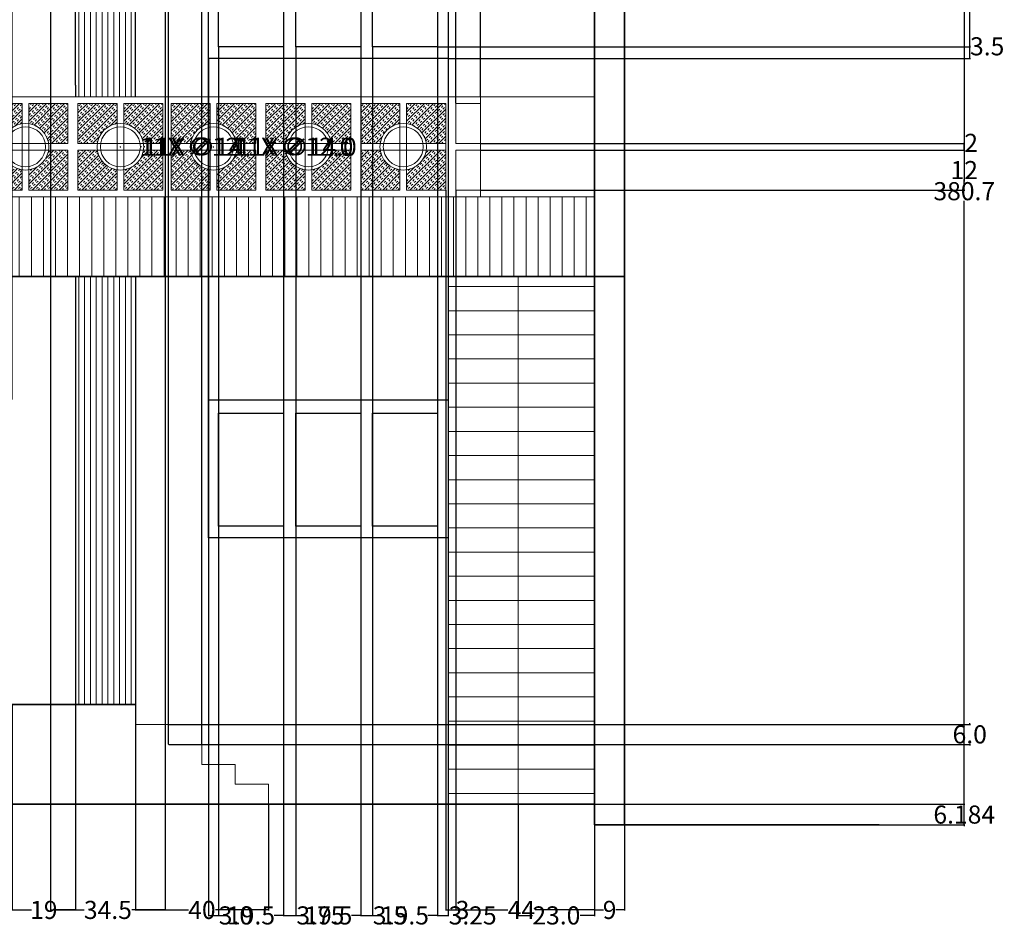
# Model space of a CAD drawing. Units: inches. Extents: x 12 to 590, y 127 to 569.
# Tile 3 of 4: x 294 to 590, y 127 to 399. Entities that reach past the tile are written whole.
import ezdxf

# ---------------------------------------------------------------- set-up
doc = ezdxf.new("R2010")
doc.units = ezdxf.units.IN
doc.header["$MEASUREMENT"] = 0
for name, color, linetype, lineweight in [('A-ANNO-DIMS', 2, 'Continuous', 18), ('A-COLS', 1, 'Continuous', 25), ('A-DETL-RAIL', 6, 'Continuous', 18), ('A-ELEV', 7, 'Continuous', 35), ('A-FLOR-STRS', 2, 'Continuous', 18), ('A-GLAZ', 4, 'Continuous', 25), ('A-WALL-PATT', 8, 'Continuous', 13)]:
    doc.layers.add(name, color=color, linetype=linetype, lineweight=lineweight)
doc.styles.get("Standard").update_dxf_attribs({"font": 'arial.ttf'})
doc.dimstyles.get("Standard").update_dxf_attribs({"dimtxt": 5.4375, "dimasz": 0.18, "dimexe": 0.18, "dimexo": 0.0625, "dimgap": 0.09, "dimtad": 0, "dimtih": 1, "dimtoh": 1, "dimdec": 4, "dimzin": 0, "dimdsep": 46, "dimlunit": 4, "dimtxsty": 'Standard', "dimcen": 0.09, "dimadec": 0, "dimazin": 0, "dimtfac": 1, "dimtdec": 4, "dimtofl": 0, "dimtmove": 0, "dimatfit": 3, "dimfxl": 1, "dimtolj": 1, "dimtzin": 0, "dimarcsym": 0})

# ---------------------------------------------------------------- blocks, each defined once
blk = doc.blocks.new('BALUSTRADE-PANEL')
for p, q in [((11.75, 13), (11.75, 26)), ((13.75, 13), (13.75, 26)), ((12.75, 14), (0, 14)), ((12.75, 12), (0, 12)), ((11.75, 13), (11.75, 0)), ((12.75, 14), (25.5, 14)), ((12.75, 12), (25.5, 12)), ((13.75, 13), (13.75, 0))]:
    blk.add_line(p, q)
for points in [[(0, 14), (0, 26), (11.75, 26)], [(13.75, 26), (25.5, 26), (25.5, 14)], [(11.75, 0), (0, 0), (0, 12)], [(25.5, 12), (25.5, 0), (13.75, 0)]]:
    blk.add_lwpolyline(points)
for radius in [7, 6]:
    blk.add_circle((12.75, 13), radius)
blk = doc.blocks.new('WIN-3PANE')
for points in [[(0, 41.5), (72, 41.5), (72, 0), (0, 0)], [(3, 37.5), (22.5, 37.5), (22.5, 3.5), (3, 3.5)], [(26.25, 37.5), (45.75, 37.5), (45.75, 3.5), (26.25, 3.5)], [(49.25, 37.5), (68.75, 37.5), (68.75, 3.5), (49.25, 3.5)]]:
    blk.add_lwpolyline(points, close=True)
blk = doc.blocks.new('*D8')
at = {"layer": 'A-ANNO-DIMS', "color": 0, "lineweight": -2, "transparency": 16777216}
for p, q in [((475.56, 538), (577.73, 538)), ((577.55, 537.82), (577.55, 350.53)), ((577.55, 157.5), (577.55, 344.79)), ((475.56, 157.32), (577.73, 157.32))]:
    blk.add_line(p, q, dxfattribs=at)
at = {"layer": 'A-ANNO-DIMS', "color": 0, "transparency": 16777216}
for points in [[(577.52, 537.82), (577.58, 537.82), (577.55, 538)], [(577.52, 157.5), (577.58, 157.5), (577.55, 157.32)]]:
    blk.add_solid(points, dxfattribs=at)
at = {"layer": 'Defpoints', "color": 0, "transparency": 16777216}
for p in [(475.5, 538), (475.5, 157.32), (577.55, 157.32)]:
    blk.add_point(p, dxfattribs=at)
at = {"layer": 'A-ANNO-DIMS', "color": 0, "transparency": 16777216, "insert": (577.55, 347.66), "char_height": 5.438, "attachment_point": 5}
blk.add_mtext('\\A1;380.7', dxfattribs=at)
blk = doc.blocks.new('*D15')
at = {"layer": 'A-ANNO-DIMS', "color": 0, "lineweight": -2, "transparency": 16777216}
for p, q in [((466.56, 163.5), (577.73, 163.5)), ((577.55, 163.68), (577.55, 163.86)), ((475.56, 157.32), (577.73, 157.32)), ((577.55, 157.14), (577.55, 156.96))]:
    blk.add_line(p, q, dxfattribs=at)
at = {"layer": 'A-ANNO-DIMS', "color": 0, "transparency": 16777216}
for points in [[(577.52, 163.68), (577.58, 163.68), (577.55, 163.5)], [(577.52, 157.14), (577.58, 157.14), (577.55, 157.32)]]:
    blk.add_solid(points, dxfattribs=at)
at = {"layer": 'Defpoints', "color": 0, "transparency": 16777216}
for p in [(466.5, 163.5), (577.55, 163.5), (475.5, 157.32)]:
    blk.add_point(p, dxfattribs=at)
at = {"layer": 'A-ANNO-DIMS', "color": 0, "transparency": 16777216, "insert": (577.55, 160.41), "char_height": 5.438, "attachment_point": 5}
blk.add_mtext('\\A1;6.184', dxfattribs=at)
blk = doc.blocks.new('*D24')
at = {"layer": 'A-ANNO-DIMS', "color": 0, "lineweight": -2, "transparency": 16777216}
for p, q in [((291.5, 193.44), (291.5, 131.59)), ((310.5, 193.44), (310.5, 131.59)), ((291.68, 131.77), (297.27, 131.77)), ((310.32, 131.77), (304.73, 131.77))]:
    blk.add_line(p, q, dxfattribs=at)
at = {"layer": 'A-ANNO-DIMS', "color": 0, "transparency": 16777216}
for points in [[(291.68, 131.8), (291.68, 131.74), (291.5, 131.77)], [(310.32, 131.8), (310.32, 131.74), (310.5, 131.77)]]:
    blk.add_solid(points, dxfattribs=at)
at = {"layer": 'Defpoints', "color": 0, "transparency": 16777216}
for p in [(291.5, 193.5), (310.5, 193.5), (310.5, 131.77)]:
    blk.add_point(p, dxfattribs=at)
at = {"layer": 'A-ANNO-DIMS', "color": 0, "transparency": 16777216, "insert": (301, 131.77), "char_height": 5.438, "attachment_point": 5}
blk.add_mtext('\\A1;19', dxfattribs=at)
blk = doc.blocks.new('*D25')
at = {"layer": 'A-ANNO-DIMS', "color": 0, "lineweight": -2, "transparency": 16777216}
for p, q in [((328.5, 193.44), (328.5, 131.59)), ((368.5, 163.44), (368.5, 131.59)), ((328.68, 131.77), (344.42, 131.77)), ((368.32, 131.77), (352.58, 131.77))]:
    blk.add_line(p, q, dxfattribs=at)
at = {"layer": 'A-ANNO-DIMS', "color": 0, "transparency": 16777216}
for points in [[(328.68, 131.8), (328.68, 131.74), (328.5, 131.77)], [(368.32, 131.8), (368.32, 131.74), (368.5, 131.77)]]:
    blk.add_solid(points, dxfattribs=at)
at = {"layer": 'Defpoints', "color": 0, "transparency": 16777216}
for p in [(328.5, 193.5), (368.5, 163.5), (368.5, 131.77)]:
    blk.add_point(p, dxfattribs=at)
at = {"layer": 'A-ANNO-DIMS', "color": 0, "transparency": 16777216, "insert": (348.5, 131.77), "char_height": 5.438, "attachment_point": 5}
blk.add_mtext('\\A1;40', dxfattribs=at)
blk = doc.blocks.new('*D26')
at = {"layer": 'A-ANNO-DIMS', "color": 0, "lineweight": -2, "transparency": 16777216}
for p, q in [((422.5, 243.44), (422.5, 131.59)), ((466.5, 163.44), (466.5, 131.59)), ((422.68, 131.77), (440.42, 131.77)), ((466.32, 131.77), (448.58, 131.77))]:
    blk.add_line(p, q, dxfattribs=at)
at = {"layer": 'A-ANNO-DIMS', "color": 0, "transparency": 16777216}
for points in [[(422.68, 131.8), (422.68, 131.74), (422.5, 131.77)], [(466.32, 131.8), (466.32, 131.74), (466.5, 131.77)]]:
    blk.add_solid(points, dxfattribs=at)
at = {"layer": 'Defpoints', "color": 0, "transparency": 16777216}
for p in [(422.5, 243.5), (466.5, 163.5), (466.5, 131.77)]:
    blk.add_point(p, dxfattribs=at)
at = {"layer": 'A-ANNO-DIMS', "color": 0, "transparency": 16777216, "insert": (444.5, 131.77), "char_height": 5.438, "attachment_point": 5}
blk.add_mtext('\\A1;44', dxfattribs=at)
blk = doc.blocks.new('*D27')
at = {"layer": 'A-ANNO-DIMS', "color": 0, "lineweight": -2, "transparency": 16777216}
for p, q in [((466.5, 163.44), (466.5, 131.59)), ((475.5, 157.25), (475.5, 131.59)), ((466.68, 131.77), (469.12, 131.77)), ((475.32, 131.77), (472.88, 131.77))]:
    blk.add_line(p, q, dxfattribs=at)
at = {"layer": 'A-ANNO-DIMS', "color": 0, "transparency": 16777216}
for points in [[(466.68, 131.8), (466.68, 131.74), (466.5, 131.77)], [(475.32, 131.8), (475.32, 131.74), (475.5, 131.77)]]:
    blk.add_solid(points, dxfattribs=at)
at = {"layer": 'Defpoints', "color": 0, "transparency": 16777216}
for p in [(466.5, 163.5), (475.5, 157.32), (475.5, 131.77)]:
    blk.add_point(p, dxfattribs=at)
at = {"layer": 'A-ANNO-DIMS', "color": 0, "transparency": 16777216, "insert": (471, 131.77), "char_height": 5.438, "attachment_point": 5}
blk.add_mtext('\\A1;9', dxfattribs=at)
blk = doc.blocks.new('*D40')
at = {"layer": 'A-ANNO-DIMS', "color": 0, "lineweight": -2, "transparency": 16777216}
for p, q in [((303, 455.94), (303, 131.59)), ((337.5, 455.94), (337.5, 131.59)), ((303.18, 131.77), (313.08, 131.77)), ((337.32, 131.77), (327.42, 131.77))]:
    blk.add_line(p, q, dxfattribs=at)
at = {"layer": 'A-ANNO-DIMS', "color": 0, "transparency": 16777216}
for points in [[(303.18, 131.8), (303.18, 131.74), (303, 131.77)], [(337.32, 131.8), (337.32, 131.74), (337.5, 131.77)]]:
    blk.add_solid(points, dxfattribs=at)
at = {"layer": 'Defpoints', "color": 0, "transparency": 16777216}
for p in [(303, 456), (337.5, 456), (337.5, 131.77)]:
    blk.add_point(p, dxfattribs=at)
at = {"layer": 'A-ANNO-DIMS', "color": 0, "transparency": 16777216, "insert": (320.25, 131.77), "char_height": 5.438, "attachment_point": 5}
blk.add_mtext('\\A1;34.5', dxfattribs=at)
blk = doc.blocks.new('*D48')
at = {"layer": 'A-ANNO-DIMS', "color": 0, "lineweight": -2, "transparency": 16777216}
for p, q in [((421.75, 347.94), (421.75, 131.59)), ((424.75, 347.94), (424.75, 131.59)), ((421.93, 131.77), (424.57, 131.77)), ((424.75, 131.77), (424.93, 131.77))]:
    blk.add_line(p, q, dxfattribs=at)
at = {"layer": 'A-ANNO-DIMS', "color": 0, "transparency": 16777216}
for points in [[(421.93, 131.8), (421.93, 131.74), (421.75, 131.77)], [(424.57, 131.8), (424.57, 131.74), (424.75, 131.77)]]:
    blk.add_solid(points, dxfattribs=at)
at = {"layer": 'Defpoints', "color": 0, "transparency": 16777216}
for p in [(421.75, 348), (424.75, 348), (424.75, 131.77)]:
    blk.add_point(p, dxfattribs=at)
at = {"layer": 'A-ANNO-DIMS', "color": 0, "transparency": 16777216, "insert": (426.8, 131.77), "char_height": 5.438, "attachment_point": 5}
blk.add_mtext('\\A1;3', dxfattribs=at)
blk = doc.blocks.new('*D49')
at = {"layer": 'A-ANNO-DIMS', "color": 0, "lineweight": -2, "transparency": 16777216}
for p, q in [((424.75, 374.06), (424.75, 563.73)), ((424.93, 563.55), (432.07, 563.55)), ((432.25, 376.06), (432.25, 563.73)), ((432.25, 563.55), (432.43, 563.55))]:
    blk.add_line(p, q, dxfattribs=at)
at = {"layer": 'A-ANNO-DIMS', "color": 0, "transparency": 16777216}
for points in [[(424.93, 563.58), (424.93, 563.52), (424.75, 563.55)], [(432.07, 563.58), (432.07, 563.52), (432.25, 563.55)]]:
    blk.add_solid(points, dxfattribs=at)
at = {"layer": 'Defpoints', "color": 0, "transparency": 16777216}
for p in [(432.25, 563.55), (432.25, 376), (424.75, 374)]:
    blk.add_point(p, dxfattribs=at)
at = {"layer": 'A-ANNO-DIMS', "color": 0, "transparency": 16777216, "insert": (437.47, 563.55), "char_height": 5.438, "attachment_point": 5}
blk.add_mtext('\\A1;7.5', dxfattribs=at)
blk = doc.blocks.new('*D50')
at = {"layer": 'A-ANNO-DIMS', "color": 0, "lineweight": -2, "transparency": 16777216}
for p, q in [((432.25, 376.06), (432.25, 563.73)), ((432.43, 563.55), (440.09, 563.55)), ((466.32, 563.55), (458.66, 563.55)), ((466.5, 376.06), (466.5, 563.73))]:
    blk.add_line(p, q, dxfattribs=at)
at = {"layer": 'A-ANNO-DIMS', "color": 0, "transparency": 16777216}
for points in [[(432.43, 563.58), (432.43, 563.52), (432.25, 563.55)], [(466.32, 563.58), (466.32, 563.52), (466.5, 563.55)]]:
    blk.add_solid(points, dxfattribs=at)
at = {"layer": 'Defpoints', "color": 0, "transparency": 16777216}
for p in [(466.5, 563.55), (432.25, 376), (466.5, 376)]:
    blk.add_point(p, dxfattribs=at)
at = {"layer": 'A-ANNO-DIMS', "color": 0, "transparency": 16777216, "insert": (449.38, 563.55), "char_height": 5.438, "attachment_point": 5}
blk.add_mtext('\\A1;34.25', dxfattribs=at)
blk = doc.blocks.new('*D51')
at = {"layer": 'A-ANNO-DIMS', "color": 0, "lineweight": -2, "transparency": 16777216}
for p, q in [((432.31, 360), (577.73, 360)), ((577.55, 359.82), (577.55, 356.82)), ((577.55, 348.18), (577.55, 351.18)), ((432.31, 348), (577.73, 348))]:
    blk.add_line(p, q, dxfattribs=at)
at = {"layer": 'A-ANNO-DIMS', "color": 0, "transparency": 16777216}
for points in [[(577.52, 359.82), (577.58, 359.82), (577.55, 360)], [(577.52, 348.18), (577.58, 348.18), (577.55, 348)]]:
    blk.add_solid(points, dxfattribs=at)
at = {"layer": 'Defpoints', "color": 0, "transparency": 16777216}
for p in [(432.25, 360), (577.55, 360), (432.25, 348)]:
    blk.add_point(p, dxfattribs=at)
at = {"layer": 'A-ANNO-DIMS', "color": 0, "transparency": 16777216, "insert": (577.55, 354), "char_height": 5.438, "attachment_point": 5}
blk.add_mtext('\\A1;12', dxfattribs=at)
blk = doc.blocks.new('*D52')
at = {"layer": 'A-ANNO-DIMS', "color": 0, "lineweight": -2, "transparency": 16777216}
for p, q in [((432.31, 362), (577.73, 362)), ((577.55, 362), (577.55, 362.18)), ((577.55, 362.18), (577.73, 362.18)), ((577.55, 360.18), (577.55, 361.82)), ((432.31, 360), (577.73, 360))]:
    blk.add_line(p, q, dxfattribs=at)
at = {"layer": 'A-ANNO-DIMS', "color": 0, "transparency": 16777216}
for points in [[(577.52, 361.82), (577.58, 361.82), (577.55, 362)], [(577.52, 360.18), (577.58, 360.18), (577.55, 360)]]:
    blk.add_solid(points, dxfattribs=at)
at = {"layer": 'Defpoints', "color": 0, "transparency": 16777216}
for p in [(432.25, 362), (577.55, 362), (432.25, 360)]:
    blk.add_point(p, dxfattribs=at)
at = {"layer": 'A-ANNO-DIMS', "color": 0, "transparency": 16777216, "insert": (579.62, 362.18), "char_height": 5.438, "attachment_point": 5}
blk.add_mtext('\\A1;2', dxfattribs=at)
blk = doc.blocks.new('*D54')
at = {"layer": 'A-ANNO-DIMS', "color": 0, "lineweight": -2, "transparency": 16777216}
for p, q in [((323.91, 361), (324.09, 361)), ((324, 360.91), (324, 361.09)), ((331.36, 361), (331.18, 361))]:
    blk.add_line(p, q, dxfattribs=at)
at = {"layer": 'A-ANNO-DIMS', "color": 0, "transparency": 16777216}
blk.add_solid([(331.18, 361.03), (331.18, 360.97), (331, 361)], dxfattribs=at)
at = {"layer": 'Defpoints', "color": 0, "transparency": 16777216}
for p in [(317, 361), (331, 361)]:
    blk.add_point(p, dxfattribs=at)
at = {"layer": 'A-ANNO-DIMS', "color": 0, "transparency": 16777216, "insert": (345.84, 361), "char_height": 5.4375, "attachment_point": 5}
blk.add_mtext('\\A1;11X ∅14', dxfattribs=at)
blk = doc.blocks.new('*D55')
at = {"layer": 'A-ANNO-DIMS', "color": 0, "lineweight": -2, "transparency": 16777216}
for p, q in [((323.91, 361), (324.09, 361)), ((324, 360.91), (324, 361.09)), ((330.36, 361), (330.18, 361))]:
    blk.add_line(p, q, dxfattribs=at)
at = {"layer": 'A-ANNO-DIMS', "color": 0, "transparency": 16777216}
blk.add_solid([(330.18, 361.03), (330.18, 360.97), (330, 361)], dxfattribs=at)
at = {"layer": 'Defpoints', "color": 0, "transparency": 16777216}
for p in [(318, 361), (330, 361)]:
    blk.add_point(p, dxfattribs=at)
at = {"layer": 'A-ANNO-DIMS', "color": 0, "transparency": 16777216, "insert": (344.83, 361), "char_height": 5.4375, "attachment_point": 5}
blk.add_mtext('\\A1;11X ∅12', dxfattribs=at)
blk = doc.blocks.new('*D60')
at = {"layer": 'A-ANNO-DIMS', "color": 0, "lineweight": -2, "transparency": 16777216}
for p, q in [((291.5, 285.06), (291.5, 565.38)), ((291.68, 565.2), (313.86, 565.2)), ((350.32, 565.2), (328.14, 565.2)), ((350.5, 285.06), (350.5, 565.38))]:
    blk.add_line(p, q, dxfattribs=at)
at = {"layer": 'A-ANNO-DIMS', "color": 0, "transparency": 16777216}
for points in [[(291.68, 565.23), (291.68, 565.17), (291.5, 565.2)], [(350.32, 565.23), (350.32, 565.17), (350.5, 565.2)]]:
    blk.add_solid(points, dxfattribs=at)
at = {"layer": 'Defpoints', "color": 0, "transparency": 16777216}
for p in [(350.5, 565.2), (291.5, 285), (350.5, 285)]:
    blk.add_point(p, dxfattribs=at)
at = {"layer": 'A-ANNO-DIMS', "color": 0, "transparency": 16777216, "insert": (321, 565.2), "char_height": 5.438, "attachment_point": 5}
blk.add_mtext('\\A1;59.0', dxfattribs=at)
blk = doc.blocks.new('*D61')
at = {"layer": 'A-ANNO-DIMS', "color": 0, "lineweight": -2, "transparency": 16777216}
for p, q in [((338.5625, 187.5), (579.38, 187.5)), ((579.2, 187.68), (579.2, 187.86)), ((338.5625, 181.5), (579.38, 181.5)), ((579.2, 181.32), (579.2, 181.14))]:
    blk.add_line(p, q, dxfattribs=at)
at = {"layer": 'A-ANNO-DIMS', "color": 0, "transparency": 16777216}
for points in [[(579.17, 187.68), (579.23, 187.68), (579.2, 187.5)], [(579.17, 181.32), (579.23, 181.32), (579.2, 181.5)]]:
    blk.add_solid(points, dxfattribs=at)
at = {"layer": 'Defpoints', "color": 0, "transparency": 16777216}
for p in [(338.5, 187.5), (338.5, 181.5), (579.2, 181.5)]:
    blk.add_point(p, dxfattribs=at)
at = {"layer": 'A-ANNO-DIMS', "color": 0, "transparency": 16777216, "insert": (579.2, 184.5), "char_height": 5.4375, "attachment_point": 5}
blk.add_mtext('\\A1;6.0', dxfattribs=at)
blk = doc.blocks.new('*D62')
at = {"layer": 'A-ANNO-DIMS', "color": 0, "lineweight": -2, "transparency": 16777216}
for p, q in [((338.5, 181.5625), (338.5, 565.38)), ((338.68, 565.2), (348.32, 565.2)), ((348.5, 181.5625), (348.5, 565.38)), ((348.5, 565.2), (348.68, 565.2))]:
    blk.add_line(p, q, dxfattribs=at)
at = {"layer": 'A-ANNO-DIMS', "color": 0, "transparency": 16777216}
for points in [[(338.68, 565.23), (338.68, 565.17), (338.5, 565.2)], [(348.32, 565.23), (348.32, 565.17), (348.5, 565.2)]]:
    blk.add_solid(points, dxfattribs=at)
at = {"layer": 'Defpoints', "color": 0, "transparency": 16777216}
for p in [(348.5, 565.2), (338.5, 181.5), (348.5, 181.5)]:
    blk.add_point(p, dxfattribs=at)
at = {"layer": 'A-ANNO-DIMS', "color": 0, "transparency": 16777216, "insert": (355.566875, 565.2), "char_height": 5.4375, "attachment_point": 5}
blk.add_mtext('\\A1;10.0', dxfattribs=at)
blk = doc.blocks.new('*D63')
at = {"layer": 'A-ANNO-DIMS', "color": 0, "lineweight": -2, "transparency": 16777216}
for p, q in [((443.5, 163.44), (443.5, 129.94)), ((466.5, 163.44), (466.5, 129.94)), ((443.68, 130.12), (447.81, 130.12)), ((466.32, 130.12), (462.19, 130.12))]:
    blk.add_line(p, q, dxfattribs=at)
at = {"layer": 'A-ANNO-DIMS', "color": 0, "transparency": 16777216}
for points in [[(443.68, 130.15), (443.68, 130.09), (443.5, 130.12)], [(466.32, 130.15), (466.32, 130.09), (466.5, 130.12)]]:
    blk.add_solid(points, dxfattribs=at)
at = {"layer": 'Defpoints', "color": 0, "transparency": 16777216}
for p in [(443.5, 163.5), (466.5, 163.5), (466.5, 130.12)]:
    blk.add_point(p, dxfattribs=at)
at = {"layer": 'A-ANNO-DIMS', "color": 0, "transparency": 16777216, "insert": (455, 130.12), "char_height": 5.438, "attachment_point": 5}
blk.add_mtext('\\A1;23.0', dxfattribs=at)
blk = doc.blocks.new('*D64')
at = {"layer": 'A-ANNO-DIMS', "color": 0, "lineweight": -2, "transparency": 16777216}
for p, q in [((353.5, 390.94), (353.5, 129.94)), ((350.5, 387.44), (350.5, 129.94)), ((350.68, 130.12), (353.32, 130.12)), ((353.5, 130.12), (353.68, 130.12))]:
    blk.add_line(p, q, dxfattribs=at)
at = {"layer": 'A-ANNO-DIMS', "color": 0, "transparency": 16777216}
for points in [[(350.68, 130.15), (350.68, 130.09), (350.5, 130.12)], [(353.32, 130.15), (353.32, 130.09), (353.5, 130.12)]]:
    blk.add_solid(points, dxfattribs=at)
at = {"layer": 'Defpoints', "color": 0, "transparency": 16777216}
for p in [(353.5, 391), (350.5, 387.5), (353.5, 130.12)]:
    blk.add_point(p, dxfattribs=at)
at = {"layer": 'A-ANNO-DIMS', "color": 0, "transparency": 16777216, "insert": (358.71, 130.12), "char_height": 5.438, "attachment_point": 5}
blk.add_mtext('\\A1;3.0', dxfattribs=at)
blk = doc.blocks.new('*D65')
at = {"layer": 'A-ANNO-DIMS', "color": 0, "lineweight": -2, "transparency": 16777216}
for p, q in [((353.5, 390.94), (353.5, 129.94)), ((373, 390.94), (373, 129.94)), ((353.68, 130.12), (356.33, 130.12)), ((372.82, 130.12), (370.17, 130.12))]:
    blk.add_line(p, q, dxfattribs=at)
at = {"layer": 'A-ANNO-DIMS', "color": 0, "transparency": 16777216}
for points in [[(353.68, 130.15), (353.68, 130.09), (353.5, 130.12)], [(372.82, 130.15), (372.82, 130.09), (373, 130.12)]]:
    blk.add_solid(points, dxfattribs=at)
at = {"layer": 'Defpoints', "color": 0, "transparency": 16777216}
for p in [(353.5, 391), (373, 391), (373, 130.12)]:
    blk.add_point(p, dxfattribs=at)
at = {"layer": 'A-ANNO-DIMS', "color": 0, "transparency": 16777216, "insert": (363.25, 130.12), "char_height": 5.438, "attachment_point": 5}
blk.add_mtext('\\A1;19.5', dxfattribs=at)
blk = doc.blocks.new('*D66')
at = {"layer": 'A-ANNO-DIMS', "color": 0, "lineweight": -2, "transparency": 16777216}
for p, q in [((373, 390.94), (373, 129.94)), ((376.75, 390.94), (376.75, 129.94)), ((373.18, 130.12), (376.57, 130.12)), ((376.75, 130.12), (376.93, 130.12))]:
    blk.add_line(p, q, dxfattribs=at)
at = {"layer": 'A-ANNO-DIMS', "color": 0, "transparency": 16777216}
for points in [[(373.18, 130.15), (373.18, 130.09), (373, 130.12)], [(376.57, 130.15), (376.57, 130.09), (376.75, 130.12)]]:
    blk.add_solid(points, dxfattribs=at)
at = {"layer": 'Defpoints', "color": 0, "transparency": 16777216}
for p in [(373, 391), (376.75, 391), (376.75, 130.12)]:
    blk.add_point(p, dxfattribs=at)
at = {"layer": 'A-ANNO-DIMS', "color": 0, "transparency": 16777216, "insert": (384.1, 130.12), "char_height": 5.438, "attachment_point": 5}
blk.add_mtext('\\A1;3.75', dxfattribs=at)
blk = doc.blocks.new('*D67')
at = {"layer": 'A-ANNO-DIMS', "color": 0, "lineweight": -2, "transparency": 16777216}
for p, q in [((376.75, 390.94), (376.75, 129.94)), ((396.25, 390.94), (396.25, 129.94)), ((376.93, 130.12), (379.58, 130.12)), ((396.07, 130.12), (393.42, 130.12))]:
    blk.add_line(p, q, dxfattribs=at)
at = {"layer": 'A-ANNO-DIMS', "color": 0, "transparency": 16777216}
for points in [[(376.93, 130.15), (376.93, 130.09), (376.75, 130.12)], [(396.07, 130.15), (396.07, 130.09), (396.25, 130.12)]]:
    blk.add_solid(points, dxfattribs=at)
at = {"layer": 'Defpoints', "color": 0, "transparency": 16777216}
for p in [(376.75, 391), (396.25, 391), (396.25, 130.12)]:
    blk.add_point(p, dxfattribs=at)
at = {"layer": 'A-ANNO-DIMS', "color": 0, "transparency": 16777216, "insert": (386.5, 130.12), "char_height": 5.438, "attachment_point": 5}
blk.add_mtext('\\A1;19.5', dxfattribs=at)
blk = doc.blocks.new('*D68')
at = {"layer": 'A-ANNO-DIMS', "color": 0, "lineweight": -2, "transparency": 16777216}
for p, q in [((396.25, 390.94), (396.25, 129.94)), ((399.75, 390.94), (399.75, 129.94)), ((396.43, 130.12), (399.57, 130.12)), ((399.75, 130.12), (399.93, 130.12))]:
    blk.add_line(p, q, dxfattribs=at)
at = {"layer": 'A-ANNO-DIMS', "color": 0, "transparency": 16777216}
for points in [[(396.43, 130.15), (396.43, 130.09), (396.25, 130.12)], [(399.57, 130.15), (399.57, 130.09), (399.75, 130.12)]]:
    blk.add_solid(points, dxfattribs=at)
at = {"layer": 'Defpoints', "color": 0, "transparency": 16777216}
for p in [(396.25, 391), (399.75, 391), (399.75, 130.12)]:
    blk.add_point(p, dxfattribs=at)
at = {"layer": 'A-ANNO-DIMS', "color": 0, "transparency": 16777216, "insert": (404.99, 130.12), "char_height": 5.438, "attachment_point": 5}
blk.add_mtext('\\A1;3.5', dxfattribs=at)
blk = doc.blocks.new('*D69')
at = {"layer": 'A-ANNO-DIMS', "color": 0, "lineweight": -2, "transparency": 16777216}
for p, q in [((399.75, 390.94), (399.75, 129.94)), ((419.25, 390.94), (419.25, 129.94)), ((399.93, 130.12), (402.58, 130.12)), ((419.07, 130.12), (416.42, 130.12))]:
    blk.add_line(p, q, dxfattribs=at)
at = {"layer": 'A-ANNO-DIMS', "color": 0, "transparency": 16777216}
for points in [[(399.93, 130.15), (399.93, 130.09), (399.75, 130.12)], [(419.07, 130.15), (419.07, 130.09), (419.25, 130.12)]]:
    blk.add_solid(points, dxfattribs=at)
at = {"layer": 'Defpoints', "color": 0, "transparency": 16777216}
for p in [(399.75, 391), (419.25, 391), (419.25, 130.12)]:
    blk.add_point(p, dxfattribs=at)
at = {"layer": 'A-ANNO-DIMS', "color": 0, "transparency": 16777216, "insert": (409.5, 130.12), "char_height": 5.438, "attachment_point": 5}
blk.add_mtext('\\A1;19.5', dxfattribs=at)
blk = doc.blocks.new('*D70')
at = {"layer": 'A-ANNO-DIMS', "color": 0, "lineweight": -2, "transparency": 16777216}
for p, q in [((419.25, 390.94), (419.25, 129.94)), ((422.5, 387.44), (422.5, 129.94)), ((419.43, 130.12), (422.32, 130.12)), ((422.5, 130.12), (422.68, 130.12))]:
    blk.add_line(p, q, dxfattribs=at)
at = {"layer": 'A-ANNO-DIMS', "color": 0, "transparency": 16777216}
for points in [[(419.43, 130.15), (419.43, 130.09), (419.25, 130.12)], [(422.32, 130.15), (422.32, 130.09), (422.5, 130.12)]]:
    blk.add_solid(points, dxfattribs=at)
at = {"layer": 'Defpoints', "color": 0, "transparency": 16777216}
for p in [(419.25, 391), (422.5, 387.5), (422.5, 130.12)]:
    blk.add_point(p, dxfattribs=at)
at = {"layer": 'A-ANNO-DIMS', "color": 0, "transparency": 16777216, "insert": (429.85, 130.12), "char_height": 5.438, "attachment_point": 5}
blk.add_mtext('\\A1;3.25', dxfattribs=at)
blk = doc.blocks.new('*D71')
at = {"layer": 'A-ANNO-DIMS', "color": 0, "lineweight": -2, "transparency": 16777216}
for p, q in [((419.31, 391), (579.38, 391)), ((579.2, 391), (579.2, 391.18)), ((579.2, 391.18), (579.38, 391.18)), ((579.2, 387.68), (579.2, 390.82)), ((422.56, 387.5), (579.38, 387.5))]:
    blk.add_line(p, q, dxfattribs=at)
at = {"layer": 'A-ANNO-DIMS', "color": 0, "transparency": 16777216}
for points in [[(579.17, 390.82), (579.23, 390.82), (579.2, 391)], [(579.17, 387.68), (579.23, 387.68), (579.2, 387.5)]]:
    blk.add_solid(points, dxfattribs=at)
at = {"layer": 'Defpoints', "color": 0, "transparency": 16777216}
for p in [(419.25, 391), (579.2, 391), (422.5, 387.5)]:
    blk.add_point(p, dxfattribs=at)
at = {"layer": 'A-ANNO-DIMS', "color": 0, "transparency": 16777216, "insert": (584.44, 391.18), "char_height": 5.438, "attachment_point": 5}
blk.add_mtext('\\A1;3.5', dxfattribs=at)
blk = doc.blocks.new('*D72')
at = {"layer": 'A-ANNO-DIMS', "color": 0, "lineweight": -2, "transparency": 16777216}
for p, q in [((419.31, 425), (579.38, 425)), ((579.2, 424.82), (579.2, 410.87)), ((579.2, 391.18), (579.2, 405.13)), ((419.31, 391), (579.38, 391))]:
    blk.add_line(p, q, dxfattribs=at)
at = {"layer": 'A-ANNO-DIMS', "color": 0, "transparency": 16777216}
for points in [[(579.17, 424.82), (579.23, 424.82), (579.2, 425)], [(579.17, 391.18), (579.23, 391.18), (579.2, 391)]]:
    blk.add_solid(points, dxfattribs=at)
at = {"layer": 'Defpoints', "color": 0, "transparency": 16777216}
for p in [(419.25, 425), (579.2, 425), (419.25, 391)]:
    blk.add_point(p, dxfattribs=at)
at = {"layer": 'A-ANNO-DIMS', "color": 0, "transparency": 16777216, "insert": (579.2, 408), "char_height": 5.438, "attachment_point": 5}
blk.add_mtext('\\A1;34.0', dxfattribs=at)
blk = doc.blocks.new('*D74')
at = {"layer": 'A-ANNO-DIMS', "color": 0, "lineweight": -2, "transparency": 16777216}
for p, q in [((351.91, 361), (352.09, 361)), ((352, 360.91), (352, 361.09)), ((359.36, 361), (359.18, 361))]:
    blk.add_line(p, q, dxfattribs=at)
at = {"layer": 'A-ANNO-DIMS', "color": 0, "transparency": 16777216}
blk.add_solid([(359.18, 361.03), (359.18, 360.97), (359, 361)], dxfattribs=at)
at = {"layer": 'Defpoints', "color": 0, "transparency": 16777216}
for p in [(345, 361), (359, 361)]:
    blk.add_point(p, dxfattribs=at)
at = {"layer": 'A-ANNO-DIMS', "color": 0, "transparency": 16777216, "insert": (377.01, 361), "char_height": 5.4375, "attachment_point": 5}
blk.add_mtext('\\A1;11X ∅14.0', dxfattribs=at)
blk = doc.blocks.new('*D75')
at = {"layer": 'A-ANNO-DIMS', "color": 0, "lineweight": -2, "transparency": 16777216}
for p, q in [((351.91, 361), (352.09, 361)), ((352, 360.91), (352, 361.09)), ((358.36, 361), (358.18, 361))]:
    blk.add_line(p, q, dxfattribs=at)
at = {"layer": 'A-ANNO-DIMS', "color": 0, "transparency": 16777216}
blk.add_solid([(358.18, 361.03), (358.18, 360.97), (358, 361)], dxfattribs=at)
at = {"layer": 'Defpoints', "color": 0, "transparency": 16777216}
for p in [(346, 361), (358, 361)]:
    blk.add_point(p, dxfattribs=at)
at = {"layer": 'A-ANNO-DIMS', "color": 0, "transparency": 16777216, "insert": (376.01, 361), "char_height": 5.4375, "attachment_point": 5}
blk.add_mtext('\\A1;11X ∅12.0', dxfattribs=at)

msp = doc.modelspace()

# ---------------------------------------------------------------- hatches: boundary and pattern name
at = {"layer": 'A-WALL-PATT'}
h = msp.add_hatch(dxfattribs=at)
h.set_pattern_fill('ANSI31', color=256, scale=14, angle=45)
h.paths.add_polyline_path([(328.5, 456), (310.5, 456), (310.5, 379.5), (310.5, 376), (328.5, 376)])
h.paths.add_polyline_path([(328.5, 322), (310.5, 322), (310.5, 193.5), (328.5, 193.5)])
h = msp.add_hatch(dxfattribs=at)
h.set_pattern_fill('INSUL', color=256, scale=5.1, angle=45)
h.set_pattern_definition([(45, (171.25, 0), (-1.352342, 1.352342), []), (45, (170.7992, 0.4508), (-1.352342, 1.352342), [0.6375, -0.6375]), (45, (170.3484, 0.9016), (-1.352342, 1.352342), [0.6375, -0.6375])])
h.paths.add_polyline_path([(294.5, 374), (282.75, 374), (282.75, 362), (288.5718, 362, -0.33252769), (294.5, 367.9282)])
h.paths.add_polyline_path([(308.25, 374), (296.5, 374), (296.5, 367.9282, -0.33252769), (302.4282, 362), (308.25, 362)])
h.paths.add_polyline_path([(308.25, 360), (302.4282, 360, -0.33252769), (296.5, 354.0718), (296.5, 348), (308.25, 348)])
h.paths.add_polyline_path([(294.5, 354.0718, -0.33252769), (288.5718, 360), (282.75, 360), (282.75, 348), (294.5, 348)])
h = msp.add_hatch(dxfattribs=at)
h.set_pattern_fill('INSUL', color=256, scale=5.1, angle=45)
h.set_pattern_definition([(45, (199.75, 0), (-1.352342, 1.352342), []), (45, (199.2992, 0.4508), (-1.352342, 1.352342), [0.6375, -0.6375]), (45, (198.8484, 0.9016), (-1.352342, 1.352342), [0.6375, -0.6375])])
h.paths.add_polyline_path([(323, 374), (311.25, 374), (311.25, 362), (317.0718, 362, -0.33252769), (323, 367.9282)])
h.paths.add_polyline_path([(336.75, 374), (325, 374), (325, 367.9282, -0.33252769), (330.9282, 362), (336.75, 362)])
h.paths.add_polyline_path([(336.75, 360), (330.9282, 360, -0.33252769), (325, 354.0718), (325, 348), (336.75, 348)])
h.paths.add_polyline_path([(323, 354.0718, -0.33252769), (317.0718, 360), (311.25, 360), (311.25, 348), (323, 348)])
h = msp.add_hatch(dxfattribs=at)
h.set_pattern_fill('INSUL', color=256, scale=5.1, angle=45)
h.set_pattern_definition([(45, (227.75, 0), (-1.352342, 1.352342), []), (45, (227.2992, 0.4508), (-1.352342, 1.352342), [0.6375, -0.6375]), (45, (226.8484, 0.9016), (-1.352342, 1.352342), [0.6375, -0.6375])])
h.paths.add_polyline_path([(351, 374), (339.25, 374), (339.25, 362), (345.0718, 362, -0.33252769), (351, 367.9282)])
h.paths.add_polyline_path([(364.75, 374), (353, 374), (353, 367.9282, -0.33252769), (358.9282, 362), (364.75, 362)])
h.paths.add_polyline_path([(364.75, 360), (358.9282, 360, -0.33252769), (353, 354.0718), (353, 348), (364.75, 348)])
h.paths.add_polyline_path([(351, 354.0718, -0.33252769), (345.0718, 360), (339.25, 360), (339.25, 348), (351, 348)])
h = msp.add_hatch(dxfattribs=at)
h.set_pattern_fill('INSUL', color=256, scale=5.1, angle=45)
h.set_pattern_definition([(45, (256.25, 0), (-1.352342, 1.352342), []), (45, (255.7992, 0.4508), (-1.352342, 1.352342), [0.6375, -0.6375]), (45, (255.3484, 0.9016), (-1.352342, 1.352342), [0.6375, -0.6375])])
h.paths.add_polyline_path([(379.5, 374), (367.75, 374), (367.75, 362), (373.5718, 362, -0.33252769), (379.5, 367.9282)])
h.paths.add_polyline_path([(393.25, 374), (381.5, 374), (381.5, 367.9282, -0.33252769), (387.4282, 362), (393.25, 362)])
h.paths.add_polyline_path([(393.25, 360), (387.4282, 360, -0.33252769), (381.5, 354.0718), (381.5, 348), (393.25, 348)])
h.paths.add_polyline_path([(379.5, 354.0718, -0.33252769), (373.5718, 360), (367.75, 360), (367.75, 348), (379.5, 348)])
h = msp.add_hatch(dxfattribs=at)
h.set_pattern_fill('INSUL', color=256, scale=5.1, angle=45)
h.set_pattern_definition([(45, (284.75, 0), (-1.352342, 1.352342), []), (45, (284.2992, 0.4508), (-1.352342, 1.352342), [0.6375, -0.6375]), (45, (283.8484, 0.9016), (-1.352342, 1.352342), [0.6375, -0.6375])])
h.paths.add_polyline_path([(408, 374), (396.25, 374), (396.25, 362), (402.0718, 362, -0.33252769), (408, 367.9282)])
h.paths.add_polyline_path([(421.75, 374), (410, 374), (410, 367.9282, -0.33252769), (415.9282, 362), (421.75, 362)])
h.paths.add_polyline_path([(421.75, 360), (415.9282, 360, -0.33252769), (410, 354.0718), (410, 348), (421.75, 348)])
h.paths.add_polyline_path([(408, 354.0718, -0.33252769), (402.0718, 360), (396.25, 360), (396.25, 348), (408, 348)])
h = msp.add_hatch(dxfattribs=at)
h.set_pattern_fill('ANSI31', color=256, scale=29, angle=45)
h.paths.add_polyline_path([(414, 322), (466.5, 322), (466.5, 346), (100.5, 346), (100.5, 322)])
h = msp.add_hatch(dxfattribs=at)
h.set_pattern_fill('ANSI31', color=256, scale=58, angle=135)
h.paths.add_polyline_path([(443.5, 322), (422.5, 322), (422.5, 163.5), (443.5, 163.5)])
h.paths.add_polyline_path([(466.5, 322), (443.5, 322), (443.5, 163.5), (466.5, 163.5)])

# ---------------------------------------------------------------- linework, layer by layer
at = {"layer": 'A-COLS'}
for p, q in [((310.5, 379.5), (310.5, 456)), ((328.5, 376), (328.5, 456)), ((310.5, 379.5), (310.5, 376)), ((310.5, 322), (310.5, 193.5)), ((328.5, 322), (328.5, 193.5))]:
    msp.add_line(p, q, dxfattribs=at)
at = {"layer": 'A-DETL-RAIL'}
for p, q in [((100.5, 376), (466.5, 376)), ((432.25, 374), (432.25, 376)), ((323, 361), (323, 374)), ((325, 361), (325, 374)), ((351, 361), (351, 374)), ((353, 361), (353, 374)), ((408, 361), (408, 374)), ((410, 361), (410, 374)), ((324, 362), (311.25, 362)), ((323, 361), (323, 348)), ((324, 362), (336.75, 362)), ((325, 361), (325, 348)), ((352, 362), (339.25, 362)), ((351, 361), (351, 348)), ((352, 362), (364.75, 362)), ((353, 361), (353, 348)), ((409, 362), (396.25, 362)), ((408, 361), (408, 348)), ((409, 362), (421.75, 362)), ((410, 361), (410, 348)), ((424.75, 362), (432.25, 362)), ((324, 360), (311.25, 360)), ((324, 360), (336.75, 360)), ((352, 360), (339.25, 360)), ((352, 360), (364.75, 360)), ((409, 360), (396.25, 360)), ((409, 360), (421.75, 360)), ((424.75, 360), (432.25, 360)), ((432.25, 348), (432.25, 346)), ((100.5, 346), (466.5, 346))]:
    msp.add_line(p, q, dxfattribs=at)
for points in [[(311.25, 362), (311.25, 374), (323, 374)], [(325, 374), (336.75, 374), (336.75, 348), (325, 348)], [(351, 348), (339.25, 348), (339.25, 374), (351, 374)], [(353, 374), (364.75, 374), (364.75, 362)], [(396.25, 362), (396.25, 374), (408, 374)], [(410, 374), (421.75, 374), (421.75, 348), (410, 348)], [(424.75, 362), (424.75, 374), (432.25, 374), (432.25, 348), (424.75, 348), (424.75, 360)], [(424.75, 374), (432.25, 374)], [(323, 348), (311.25, 348), (311.25, 360)], [(364.75, 360), (364.75, 348), (353, 348)], [(408, 348), (396.25, 348), (396.25, 360)], [(432.25, 348), (424.75, 348)]]:
    msp.add_lwpolyline(points, dxfattribs=at)
for centre, radius in [((324, 361), 7), ((324, 361), 6), ((352, 361), 7), ((352, 361), 6), ((409, 361), 7), ((409, 361), 6)]:
    msp.add_circle(centre, radius, dxfattribs=at)
at = {"layer": 'A-ELEV'}
for p, q in [((475.5, 322), (475.5, 484.5)), ((466.5, 322), (466.5, 466)), ((100.5, 322), (414, 322)), ((414, 322), (475.5, 322)), ((466.5, 322), (466.5, 163.5)), ((475.5, 322), (475.5, 163.5)), ((100.5, 193.5), (328.5, 193.5)), ((100.5, 163.5), (422, 163.5)), ((422, 163.5), (466.5, 163.5)), ((466.5, 163.5), (466.5, 157.3163)), ((475.5, 163.5), (475.5, 157.3163)), ((466.5, 157.3163), (552, 157.3163))]:
    msp.add_line(p, q, dxfattribs=at)
at = {"layer": 'A-FLOR-STRS'}
for p, q in [((422.5, 322), (422.5, 163.5)), ((443.5, 322), (443.5, 163.5)), ((328.5, 193.5), (328.5, 187.5)), ((328.5, 187.5), (338.5, 187.5)), ((338.5, 187.5), (338.5, 181.5)), ((338.5, 181.5), (348.5, 181.5)), ((348.5, 181.5), (348.5, 175.5)), ((348.5, 175.5), (358.5, 175.5)), ((358.5, 175.5), (358.5, 169.5)), ((358.5, 169.5), (368.5, 169.5)), ((368.5, 169.5), (368.5, 163.5))]:
    msp.add_line(p, q, dxfattribs=at)

# ---------------------------------------------------------------- block references
at = {"layer": 'A-DETL-RAIL'}
msp.add_blockref('BALUSTRADE-PANEL', (282.75, 348), dxfattribs=at)
at = {"layer": 'A-DETL-RAIL', "rotation": 180}
msp.add_blockref('BALUSTRADE-PANEL', (393.25, 374), dxfattribs=at)
at = {"layer": 'A-GLAZ'}
for p in [(350.5, 387.5), (350.5, 243.5)]:
    msp.add_blockref('WIN-3PANE', p, dxfattribs=at)

# ---------------------------------------------------------------- dimensions: what is measured, and where the dimension line sits
at = {"layer": 'A-ANNO-DIMS'}
for base, p1, p2, override, picture, middle in [((350.5, 565.2), (291.5, 285), (350.5, 285), {"dimdec": 1, "dimlfac": 1, "dimrnd": 0, "dimzin": 0, "dimdsep": 46, "dimlunit": 2}, '*D60', (321, 565.2)), ((348.5, 565.2), (338.5, 181.5), (348.5, 181.5), {"dimdec": 1, "dimlfac": 1, "dimrnd": 0, "dimzin": 0, "dimdsep": 46, "dimlunit": 2}, '*D62', (355.5669, 565.2)), ((432.25, 563.55), (424.75, 374), (432.25, 376), {"dimdec": 1, "dimlfac": 1, "dimrnd": 0, "dimzin": 0, "dimdsep": 46, "dimlunit": 2}, '*D49', (437.4679, 563.55)), ((466.5, 563.55), (432.25, 376), (466.5, 376), {"dimdec": 2, "dimlfac": 1, "dimrnd": 0, "dimzin": 0, "dimdsep": 46, "dimlunit": 2}, '*D50', (449.375, 563.55)), ((337.5, 131.7663), (303, 456), (337.5, 456), {"dimdec": 1, "dimlfac": 1, "dimrnd": 0, "dimzin": 0, "dimdsep": 46, "dimlunit": 2}, '*D40', (320.25, 131.7663)), ((353.5, 130.1163), (350.5, 387.5), (353.5, 391), {"dimdec": 1, "dimlfac": 1, "dimrnd": 0, "dimzin": 0, "dimdsep": 46, "dimlunit": 2}, '*D64', (358.7086, 130.1163)), ((373, 130.1163), (353.5, 391), (373, 391), {"dimdec": 1, "dimlfac": 1, "dimrnd": 0, "dimzin": 0, "dimdsep": 46, "dimlunit": 2}, '*D65', (363.25, 130.1163)), ((376.75, 130.1163), (373, 391), (376.75, 391), {"dimdec": 2, "dimlfac": 1, "dimrnd": 0, "dimzin": 0, "dimdsep": 46, "dimlunit": 2}, '*D66', (384.1006, 130.1163)), ((396.25, 130.1163), (376.75, 391), (396.25, 391), {"dimdec": 1, "dimlfac": 1, "dimrnd": 0, "dimzin": 0, "dimdsep": 46, "dimlunit": 2}, '*D67', (386.5, 130.1163)), ((399.75, 130.1163), (396.25, 391), (399.75, 391), {"dimdec": 1, "dimlfac": 1, "dimrnd": 0, "dimzin": 0, "dimdsep": 46, "dimlunit": 2}, '*D68', (404.9883, 130.1163)), ((419.25, 130.1163), (399.75, 391), (419.25, 391), {"dimdec": 1, "dimlfac": 1, "dimrnd": 0, "dimzin": 0, "dimdsep": 46, "dimlunit": 2}, '*D69', (409.5, 130.1163)), ((422.5, 130.1163), (419.25, 391), (422.5, 387.5), {"dimdec": 2, "dimlfac": 1, "dimrnd": 0, "dimzin": 0, "dimdsep": 46, "dimlunit": 2}, '*D70', (429.8506, 130.1163)), ((424.75, 131.7663), (421.75, 348), (424.75, 348), {"dimdec": 0, "dimlfac": 1, "dimrnd": 0, "dimzin": 0, "dimdsep": 46, "dimlunit": 2}, '*D48', (426.8004, 131.7663)), ((466.5, 131.7663), (422.5, 243.5), (466.5, 163.5), {"dimdec": 0, "dimlfac": 1, "dimrnd": 0, "dimzin": 0, "dimdsep": 46, "dimlunit": 2}, '*D26', (444.5, 131.7663)), ((310.5, 131.7663), (291.5, 193.5), (310.5, 193.5), {"dimdec": 0, "dimlfac": 1, "dimrnd": 0, "dimzin": 0, "dimdsep": 46, "dimlunit": 2}, '*D24', (301, 131.7663)), ((368.5, 131.7663), (328.5, 193.5), (368.5, 163.5), {"dimdec": 0, "dimlfac": 1, "dimrnd": 0, "dimzin": 0, "dimdsep": 46, "dimlunit": 2}, '*D25', (348.5, 131.7663)), ((466.5, 130.1163), (443.5, 163.5), (466.5, 163.5), {"dimdec": 1, "dimlfac": 1, "dimrnd": 0, "dimzin": 0, "dimdsep": 46, "dimlunit": 2}, '*D63', (455, 130.1163)), ((475.5, 131.7663), (466.5, 163.5), (475.5, 157.3163), {"dimdec": 0, "dimlfac": 1, "dimrnd": 0, "dimzin": 0, "dimdsep": 46, "dimlunit": 2}, '*D27', (471, 131.7663))]:
    dim = msp.add_linear_dim(base=base, p1=p1, p2=p2, dimstyle='Standard', override=override, dxfattribs=at)
    dim.commit()
    dim.dimension.update_dxf_attribs({"geometry": picture, "text_midpoint": middle})
for base, p1, p2, override, picture, middle in [((577.55, 157.3163), (475.5, 538), (475.5, 157.3163), {"dimdec": 1, "dimlfac": 1, "dimrnd": 0, "dimzin": 0, "dimdsep": 46, "dimlunit": 2}, '*D8', (577.55, 347.6581)), ((579.2, 425), (419.25, 391), (419.25, 425), {"dimdec": 1, "dimlfac": 1, "dimrnd": 0, "dimzin": 0, "dimdsep": 46, "dimlunit": 2}, '*D72', (579.2, 408)), ((579.2, 391), (422.5, 387.5), (419.25, 391), {"dimdec": 1, "dimlfac": 1, "dimrnd": 0, "dimzin": 0, "dimdsep": 46, "dimlunit": 2}, '*D71', (584.4383, 391.18)), ((577.55, 362), (432.25, 360), (432.25, 362), {"dimdec": 0, "dimlfac": 1, "dimrnd": 0, "dimzin": 0, "dimdsep": 46, "dimlunit": 2}, '*D52', (579.6208, 362.18)), ((577.55, 360), (432.25, 348), (432.25, 360), {"dimdec": 0, "dimlfac": 1, "dimrnd": 0, "dimzin": 0, "dimdsep": 46, "dimlunit": 2}, '*D51', (577.55, 354)), ((579.2, 181.5), (338.5, 187.5), (338.5, 181.5), {"dimdec": 1, "dimlfac": 1, "dimrnd": 0, "dimzin": 0, "dimdsep": 46, "dimlunit": 2}, '*D61', (579.2, 184.5)), ((577.55, 163.5), (475.5, 157.3163), (466.5, 163.5), {"dimdec": 3, "dimlfac": 1, "dimrnd": 0, "dimzin": 0, "dimdsep": 46, "dimlunit": 2}, '*D15', (577.55, 160.4081))]:
    dim = msp.add_linear_dim(base=base, p1=p1, p2=p2, angle=90, dimstyle='Standard', override=override, dxfattribs=at)
    dim.commit()
    dim.dimension.update_dxf_attribs({"geometry": picture, "text_midpoint": middle})
dim = msp.add_diameter_dim_2p(p1=(317, 361), p2=(331, 361), text='11X <>', dimstyle='Standard', override={"dimdec": 0, "dimlfac": 1, "dimrnd": 0, "dimzin": 0, "dimdsep": 46, "dimlunit": 2}, dxfattribs=at)
dim.commit()
dim.dimension.update_dxf_attribs({"geometry": '*D54', "text_midpoint": (345.8449, 361)})
for p1, p2, override, picture, middle in [((318, 361), (330, 361), {"dimdec": 0, "dimlfac": 1, "dimrnd": 0, "dimzin": 0, "dimdsep": 46, "dimlunit": 2}, '*D55', (344.8282, 361)), ((345, 361), (359, 361), {"dimdec": 1, "dimlfac": 1, "dimrnd": 0, "dimzin": 0, "dimdsep": 46, "dimlunit": 2}, '*D74', (377.0143, 361)), ((346, 361), (358, 361), {"dimdec": 1, "dimlfac": 1, "dimrnd": 0, "dimzin": 0, "dimdsep": 46, "dimlunit": 2}, '*D75', (376.0143, 361))]:
    dim = msp.add_diameter_dim_2p(p1=p1, p2=p2, text='11X <>', dimstyle='Standard', override=override, dxfattribs=at)
    dim.commit()
    dim.dimension.update_dxf_attribs({"geometry": picture, "text_midpoint": middle, "dimtype": 163})

doc.saveas('drawing.dxf')
